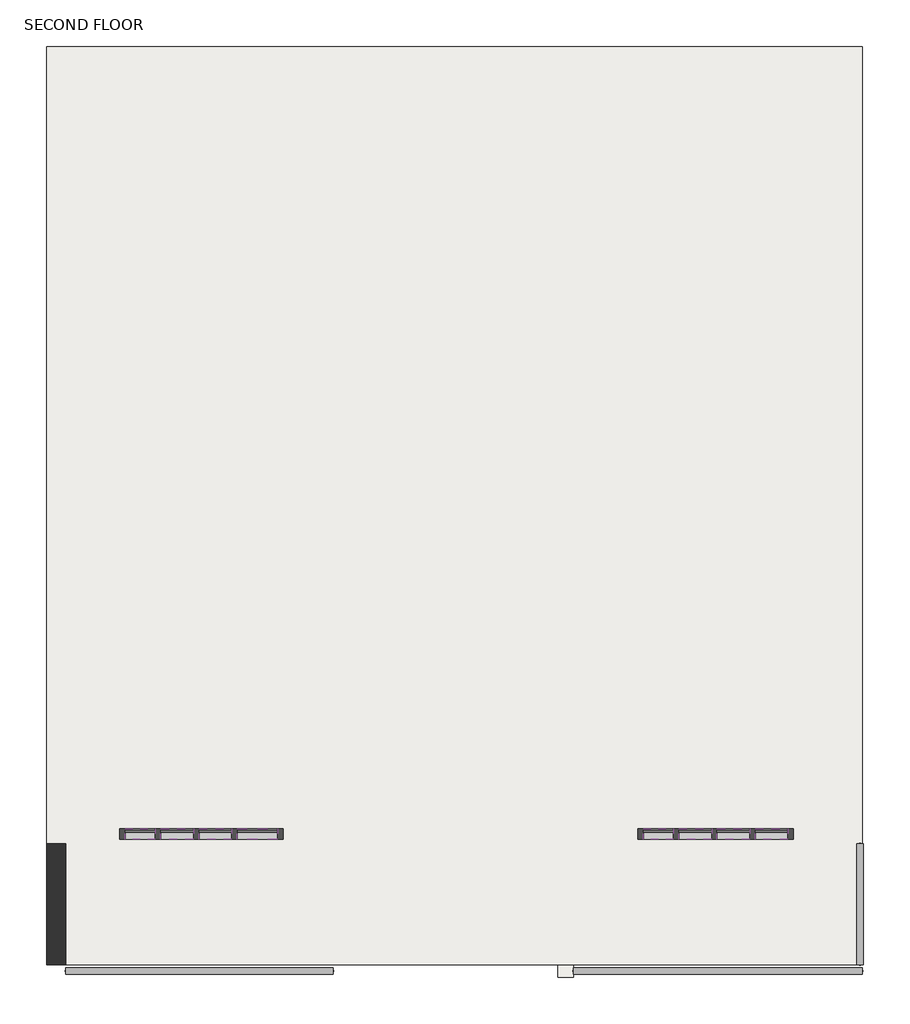
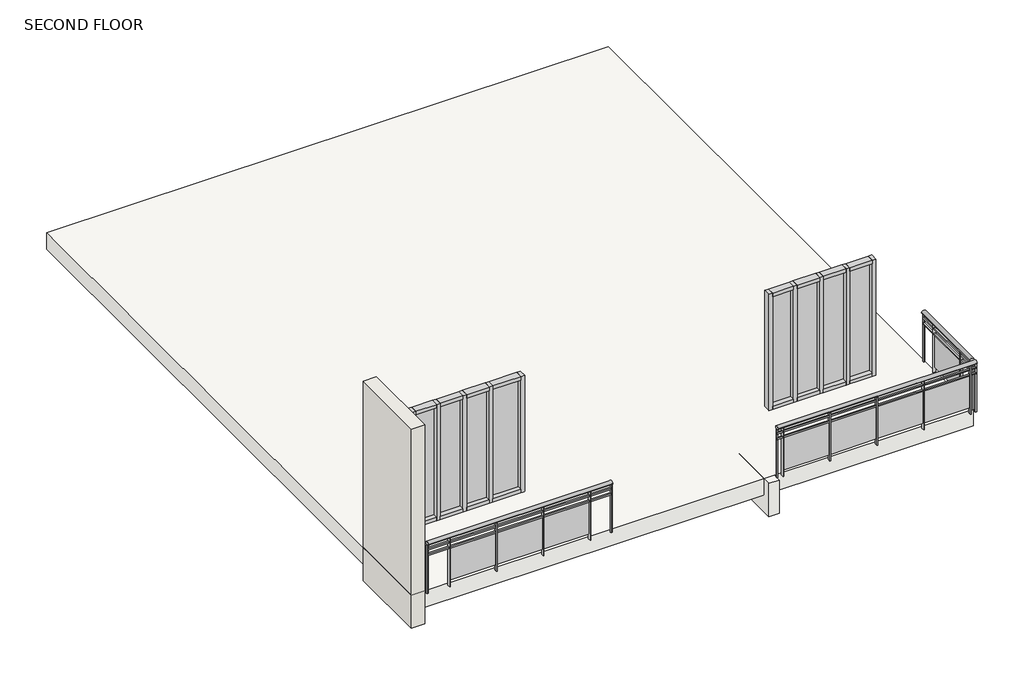
# One storey: 26 members, 8 plates, 3 railings, 2 slabs, 1 wall.
"""IFC4 building model written with IfcOpenShell, lengths in millimetres."""

from ifc_helpers import new_model, si_unit, point, frame, origin, place, context, project, spatial, polyline, ellipse_curve, trimmed, outline, extrude, transform, mapped, element, save
from ifc_brep_helpers import plane_surface, extruded_surface, advanced_brep
from components import member_3374d9b6, member_7cbddb58, member_843225dc, member_7096a90e, member_499db0bc, member_75a0f14a, system_panel_glazed_935821d8, system_panel_glazed_f3f5655f, system_panel_glazed_1490133a, system_panel_glazed_451412b5, floors_3_floors_3_f25fb9f3

model = new_model("IFC4")

# Units and contexts
model_context = context("Model", 3, world=origin())
ifc_project = project(units=[si_unit("LENGTHUNIT", "METRE", prefix="MILLI")], contexts=[model_context])

# Site, building, storey
site = spatial("IfcSite", under=ifc_project)
building = spatial("IfcBuilding", under=site)
storey = spatial("IfcBuildingStorey", under=building, Name="SECOND FLOOR", Elevation=6096.0)

# Members
placement = place(None, origin())
member_shape = member_3374d9b6(model_context)
element("IfcMember", 1, ObjectType="Rectangular Mullion : 2.5\" x 5\" rectangular", at=placement, inside=storey, context=model_context, shape_type="MappedRepresentation", body=[
    mapped(member_shape, transform((-3493.058803, -508.3464931, 6096.0), x_axis=(1.0, 0.0, 0.0), y_axis=(0.0, -1.0, 0.0), z_axis=(0.0, 0.0, -1.0))),
])
element("IfcMember", 2, ObjectType="Rectangular Mullion : 2.5\" x 5\" rectangular", at=placement, inside=storey, context=model_context, shape_type="MappedRepresentation", body=[
    mapped(member_shape, transform((2606.0769214, -508.3464931, 6096.0), x_axis=(1.0, 0.0, 0.0), y_axis=(0.0, -1.0, 0.0), z_axis=(0.0, 0.0, -1.0))),
])
element("IfcMember", 3, ObjectType="Rectangular Mullion : 2.5\" x 5\" rectangular", at=placement, inside=storey, context=model_context, shape_type="MappedRepresentation", body=[
    mapped(member_shape, transform((-5445.7230786, -508.3464931, 8229.6), x_axis=(-1.0, 0.0, 0.0), y_axis=(0.0, -1.0, 0.0), z_axis=(0.0, 0.0, 1.0))),
])
element("IfcMember", 4, ObjectType="Rectangular Mullion : 2.5\" x 5\" rectangular", at=placement, inside=storey, context=model_context, shape_type="MappedRepresentation", body=[
    mapped(member_shape, transform((748.741197, -508.3464931, 8229.6), x_axis=(-1.0, 0.0, 0.0), y_axis=(0.0, -1.0, 0.0), z_axis=(0.0, 0.0, 1.0))),
])
member_2_shape = member_7cbddb58(model_context)
element("IfcMember", 5, ObjectType="Rectangular Mullion : 2.5\" x 5\" rectangular", at=placement, inside=storey, context=model_context, shape_type="MappedRepresentation", body=[
    mapped(member_2_shape, transform((-4988.5230786, -508.3464931, 6096.0), x_axis=(1.0, 0.0, 0.0), y_axis=(0.0, -1.0, 0.0), z_axis=(0.0, 0.0, -1.0))),
])
element("IfcMember", 6, ObjectType="Rectangular Mullion : 2.5\" x 5\" rectangular", at=placement, inside=storey, context=model_context, shape_type="MappedRepresentation", body=[
    mapped(member_2_shape, transform((-4531.3230786, -508.3464931, 6096.0), x_axis=(1.0, 0.0, 0.0), y_axis=(0.0, -1.0, 0.0), z_axis=(0.0, 0.0, -1.0))),
])
element("IfcMember", 7, ObjectType="Rectangular Mullion : 2.5\" x 5\" rectangular", at=placement, inside=storey, context=model_context, shape_type="MappedRepresentation", body=[
    mapped(member_2_shape, transform((-4074.1230786, -508.3464931, 6096.0), x_axis=(1.0, 0.0, 0.0), y_axis=(0.0, -1.0, 0.0), z_axis=(0.0, 0.0, -1.0))),
])
element("IfcMember", 8, ObjectType="Rectangular Mullion : 2.5\" x 5\" rectangular", at=placement, inside=storey, context=model_context, shape_type="MappedRepresentation", body=[
    mapped(member_2_shape, transform((1205.941197, -508.3464931, 6096.0), x_axis=(1.0, 0.0, 0.0), y_axis=(0.0, -1.0, 0.0), z_axis=(0.0, 0.0, -1.0))),
])
element("IfcMember", 9, ObjectType="Rectangular Mullion : 2.5\" x 5\" rectangular", at=placement, inside=storey, context=model_context, shape_type="MappedRepresentation", body=[
    mapped(member_2_shape, transform((1663.141197, -508.3464931, 6096.0), x_axis=(1.0, 0.0, 0.0), y_axis=(0.0, -1.0, 0.0), z_axis=(0.0, 0.0, -1.0))),
])
element("IfcMember", 10, ObjectType="Rectangular Mullion : 2.5\" x 5\" rectangular", at=placement, inside=storey, context=model_context, shape_type="MappedRepresentation", body=[
    mapped(member_2_shape, transform((2120.341197, -508.3464931, 6096.0), x_axis=(1.0, 0.0, 0.0), y_axis=(0.0, -1.0, 0.0), z_axis=(0.0, 0.0, -1.0))),
])
member_3_shape = member_843225dc(model_context)
element("IfcMember", 11, ObjectType="Rectangular Mullion : 2.5\" x 5\" rectangular", at=placement, inside=storey, context=model_context, shape_type="MappedRepresentation", body=[
    mapped(member_3_shape, transform((-5382.2230786, -508.3464931, 6096.0), x_axis=(0.0, 0.0, -1.0), y_axis=(0.0, -1.0, 0.0), z_axis=(-1.0, 0.0, 0.0))),
])
element("IfcMember", 12, ObjectType="Rectangular Mullion : 2.5\" x 5\" rectangular", at=placement, inside=storey, context=model_context, shape_type="MappedRepresentation", body=[
    mapped(member_3_shape, transform((812.241197, -508.3464931, 6096.0), x_axis=(0.0, 0.0, -1.0), y_axis=(0.0, -1.0, 0.0), z_axis=(-1.0, 0.0, 0.0))),
])
element("IfcMember", 13, ObjectType="Rectangular Mullion : 2.5\" x 5\" rectangular", at=placement, inside=storey, context=model_context, shape_type="MappedRepresentation", body=[
    mapped(member_3_shape, transform((-5020.2730786, -508.3464931, 8229.6), x_axis=(0.0, 0.0, 1.0), y_axis=(0.0, -1.0, 0.0), z_axis=(1.0, 0.0, 0.0))),
])
element("IfcMember", 14, ObjectType="Rectangular Mullion : 2.5\" x 5\" rectangular", at=placement, inside=storey, context=model_context, shape_type="MappedRepresentation", body=[
    mapped(member_3_shape, transform((1174.191197, -508.3464931, 8229.6), x_axis=(0.0, 0.0, 1.0), y_axis=(0.0, -1.0, 0.0), z_axis=(1.0, 0.0, 0.0))),
])
member_4_shape = member_7096a90e(model_context)
element("IfcMember", 15, ObjectType="Rectangular Mullion : 2.5\" x 5\" rectangular", at=placement, inside=storey, context=model_context, shape_type="MappedRepresentation", body=[
    mapped(member_4_shape, transform((-4956.7730786, -508.3464931, 6096.0), x_axis=(0.0, 0.0, -1.0), y_axis=(0.0, -1.0, 0.0), z_axis=(-1.0, 0.0, 0.0))),
])
element("IfcMember", 16, ObjectType="Rectangular Mullion : 2.5\" x 5\" rectangular", at=placement, inside=storey, context=model_context, shape_type="MappedRepresentation", body=[
    mapped(member_4_shape, transform((-4499.5730786, -508.3464931, 6096.0), x_axis=(0.0, 0.0, -1.0), y_axis=(0.0, -1.0, 0.0), z_axis=(-1.0, 0.0, 0.0))),
])
element("IfcMember", 17, ObjectType="Rectangular Mullion : 2.5\" x 5\" rectangular", at=placement, inside=storey, context=model_context, shape_type="MappedRepresentation", body=[
    mapped(member_4_shape, transform((1237.691197, -508.3464931, 6096.0), x_axis=(0.0, 0.0, -1.0), y_axis=(0.0, -1.0, 0.0), z_axis=(-1.0, 0.0, 0.0))),
])
element("IfcMember", 18, ObjectType="Rectangular Mullion : 2.5\" x 5\" rectangular", at=placement, inside=storey, context=model_context, shape_type="MappedRepresentation", body=[
    mapped(member_4_shape, transform((1694.891197, -508.3464931, 6096.0), x_axis=(0.0, 0.0, -1.0), y_axis=(0.0, -1.0, 0.0), z_axis=(-1.0, 0.0, 0.0))),
])
element("IfcMember", 19, ObjectType="Rectangular Mullion : 2.5\" x 5\" rectangular", at=placement, inside=storey, context=model_context, shape_type="MappedRepresentation", body=[
    mapped(member_4_shape, transform((-4563.0730786, -508.3464931, 8229.6), x_axis=(0.0, 0.0, 1.0), y_axis=(0.0, -1.0, 0.0), z_axis=(1.0, 0.0, 0.0))),
])
element("IfcMember", 20, ObjectType="Rectangular Mullion : 2.5\" x 5\" rectangular", at=placement, inside=storey, context=model_context, shape_type="MappedRepresentation", body=[
    mapped(member_4_shape, transform((-4105.8730786, -508.3464931, 8229.6), x_axis=(0.0, 0.0, 1.0), y_axis=(0.0, -1.0, 0.0), z_axis=(1.0, 0.0, 0.0))),
])
element("IfcMember", 21, ObjectType="Rectangular Mullion : 2.5\" x 5\" rectangular", at=placement, inside=storey, context=model_context, shape_type="MappedRepresentation", body=[
    mapped(member_4_shape, transform((1631.391197, -508.3464931, 8229.6), x_axis=(0.0, 0.0, 1.0), y_axis=(0.0, -1.0, 0.0), z_axis=(1.0, 0.0, 0.0))),
])
element("IfcMember", 22, ObjectType="Rectangular Mullion : 2.5\" x 5\" rectangular", at=placement, inside=storey, context=model_context, shape_type="MappedRepresentation", body=[
    mapped(member_4_shape, transform((2088.591197, -508.3464931, 8229.6), x_axis=(0.0, 0.0, 1.0), y_axis=(0.0, -1.0, 0.0), z_axis=(1.0, 0.0, 0.0))),
])
member_5_shape = member_499db0bc(model_context)
element("IfcMember", 23, ObjectType="Rectangular Mullion : 2.5\" x 5\" rectangular", at=placement, inside=storey, context=model_context, shape_type="MappedRepresentation", body=[
    mapped(member_5_shape, transform((-3556.558803, -508.3464931, 8229.6), x_axis=(0.0, 0.0, 1.0), y_axis=(0.0, -1.0, 0.0), z_axis=(1.0, 0.0, 0.0))),
])
element("IfcMember", 24, ObjectType="Rectangular Mullion : 2.5\" x 5\" rectangular", at=placement, inside=storey, context=model_context, shape_type="MappedRepresentation", body=[
    mapped(member_5_shape, transform((-4042.3730786, -508.3464931, 6096.0), x_axis=(0.0, 0.0, -1.0), y_axis=(0.0, -1.0, 0.0), z_axis=(-1.0, 0.0, 0.0))),
])
member_6_shape = member_75a0f14a(model_context)
element("IfcMember", 25, ObjectType="Rectangular Mullion : 2.5\" x 5\" rectangular", at=placement, inside=storey, context=model_context, shape_type="MappedRepresentation", body=[
    mapped(member_6_shape, transform((2542.5769214, -508.3464931, 8229.6), x_axis=(0.0, 0.0, 1.0), y_axis=(0.0, -1.0, 0.0), z_axis=(1.0, 0.0, 0.0))),
])
element("IfcMember", 26, ObjectType="Rectangular Mullion : 2.5\" x 5\" rectangular", at=placement, inside=storey, context=model_context, shape_type="MappedRepresentation", body=[
    mapped(member_6_shape, transform((2152.091197, -508.3464931, 6096.0), x_axis=(0.0, 0.0, -1.0), y_axis=(0.0, -1.0, 0.0), z_axis=(-1.0, 0.0, 0.0))),
])

# Plates
system_panel_glazed_shape = system_panel_glazed_935821d8(model_context)
element("IfcPlate", 27, ObjectType="System Panel : Glazed", at=placement, inside=storey, context=model_context, shape_type="MappedRepresentation", body=[
    mapped(system_panel_glazed_shape, transform((-5201.2480786, -508.3464931, 6159.5), x_axis=(1.0, 0.0, 0.0), y_axis=(0.0, 1.0, 0.0), z_axis=(0.0, 0.0, 1.0))),
])
element("IfcPlate", 28, ObjectType="System Panel : Glazed", at=placement, inside=storey, context=model_context, shape_type="MappedRepresentation", body=[
    mapped(system_panel_glazed_shape, transform((993.216197, -508.3464931, 6159.5), x_axis=(1.0, 0.0, 0.0), y_axis=(0.0, 1.0, 0.0), z_axis=(0.0, 0.0, 1.0))),
])
system_panel_glazed_2_shape = system_panel_glazed_f3f5655f(model_context)
element("IfcPlate", 29, ObjectType="System Panel : Glazed", at=placement, inside=storey, context=model_context, shape_type="MappedRepresentation", body=[
    mapped(system_panel_glazed_2_shape, transform((-4759.9230786, -508.3464931, 6159.5), x_axis=(1.0, 0.0, 0.0), y_axis=(0.0, 1.0, 0.0), z_axis=(0.0, 0.0, 1.0))),
])
element("IfcPlate", 30, ObjectType="System Panel : Glazed", at=placement, inside=storey, context=model_context, shape_type="MappedRepresentation", body=[
    mapped(system_panel_glazed_2_shape, transform((-4302.7230786, -508.3464931, 6159.5), x_axis=(1.0, 0.0, 0.0), y_axis=(0.0, 1.0, 0.0), z_axis=(0.0, 0.0, 1.0))),
])
element("IfcPlate", 31, ObjectType="System Panel : Glazed", at=placement, inside=storey, context=model_context, shape_type="MappedRepresentation", body=[
    mapped(system_panel_glazed_2_shape, transform((1434.541197, -508.3464931, 6159.5), x_axis=(1.0, 0.0, 0.0), y_axis=(0.0, 1.0, 0.0), z_axis=(0.0, 0.0, 1.0))),
])
element("IfcPlate", 32, ObjectType="System Panel : Glazed", at=placement, inside=storey, context=model_context, shape_type="MappedRepresentation", body=[
    mapped(system_panel_glazed_2_shape, transform((1891.741197, -508.3464931, 6159.5), x_axis=(1.0, 0.0, 0.0), y_axis=(0.0, 1.0, 0.0), z_axis=(0.0, 0.0, 1.0))),
])
system_panel_glazed_3_shape = system_panel_glazed_1490133a(model_context)
element("IfcPlate", 33, ObjectType="System Panel : Glazed", at=placement, inside=storey, context=model_context, shape_type="MappedRepresentation", body=[
    mapped(system_panel_glazed_3_shape, transform((-3799.4659408, -508.3464931, 6159.5), x_axis=(1.0, 0.0, 0.0), y_axis=(0.0, 1.0, 0.0), z_axis=(0.0, 0.0, 1.0))),
])
system_panel_glazed_4_shape = system_panel_glazed_451412b5(model_context)
element("IfcPlate", 34, ObjectType="System Panel : Glazed", at=placement, inside=storey, context=model_context, shape_type="MappedRepresentation", body=[
    mapped(system_panel_glazed_4_shape, transform((2347.3340592, -508.3464931, 6159.5), x_axis=(1.0, 0.0, 0.0), y_axis=(0.0, 1.0, 0.0), z_axis=(0.0, 0.0, 1.0))),
])

# Railings
element("IfcRailing", 35, ObjectType="Glass Panel - Bottom Fill", at=placement, inside=storey, context=model_context, shape_type="SolidModel", body=[
    advanced_brep(
    [(-6093.4230786, -2108.5464178, 7010.4), (-6093.4230786, -2184.7464178, 7010.4), (-2893.0230786, -2108.5464178, 7010.4), (-2893.0230786, -2184.7464178, 7010.4)],
    [
        (0, 1, ellipse_curve(frame((-6093.4230786, -2146.6464178, 7010.4), z_axis=(-1.0, 0.0, 0.0), x_axis=(0.0, -1.0, 0.0)), 38.1, 28.575)),
        (1, 0, ellipse_curve(frame((-6093.4230786, -2146.6464178, 7010.4), z_axis=(-1.0, 0.0, 0.0), x_axis=(0.0, -1.0, 0.0)), 38.1, 28.575)),
        (2, 3, ellipse_curve(frame((-2893.0230786, -2146.6464178, 7010.4), z_axis=(1.0, 0.0, 0.0), x_axis=(0.0, -1.0, 0.0)), 38.1, 28.575)),
        (3, 2, ellipse_curve(frame((-2893.0230786, -2146.6464178, 7010.4), z_axis=(1.0, 0.0, 0.0), x_axis=(0.0, -1.0, 0.0)), 38.1, 28.575)),
        (0, 2),
        (3, 1),
    ],
    [
        plane_surface(frame((-6093.4230786, -2146.6464178, 7010.4), z_axis=(-1.0, 0.0, 0.0), x_axis=(0.0, 1.0, 0.0))),
        plane_surface(frame((-2893.0230786, -2146.6464178, 7010.4), z_axis=(1.0, 0.0, 0.0), x_axis=(0.0, 1.0, 0.0))),
        extruded_surface(trimmed(ellipse_curve(frame((-2893.0230786, -2146.6464178, 7010.4), z_axis=(-1.0, 0.0, 0.0), x_axis=(0.0, -1.0, 0.0)), 38.1, 28.575), [point((-2893.0230786, -2108.5464178, 7010.4))], [point((-2893.0230786, -2184.7464178, 7010.4))], True, "CARTESIAN"), (-3200.3999999999996, 0.0, 0.0), 3200.3999999999996),
        extruded_surface(trimmed(ellipse_curve(frame((-2893.0230786, -2146.6464178, 7010.4), z_axis=(-1.0, 0.0, 0.0), x_axis=(0.0, -1.0, 0.0)), 38.1, 28.575), [point((-2893.0230786, -2184.7464178, 7010.4))], [point((-2893.0230786, -2108.5464178, 7010.4))], True, "CARTESIAN"), (-3200.3999999999996, 0.0, 0.0), 3200.3999999999996),
    ],
    [
        (0, [[1, 2]]),
        (1, [[3, 4]]),
        (2, [[-1, 5, -4, 6]]),
        (3, [[-2, -6, -3, -5]]),
    ],
),
    extrude(outline(polyline([(-6093.4230786, -2159.3464178), (-6093.4230786, -2133.9464178), (-2893.0230786, -2133.9464178), (-2893.0230786, -2159.3464178), (-6093.4230786, -2159.3464178)])), frame((0.0, 0.0, 6896.1), z_axis=(0.0, 0.0, 1.0), x_axis=(1.0, 0.0, 0.0)), (0.0, 0.0, 1.0), 25.4),
    extrude(outline(polyline([(-6093.4230786, -2159.3464178), (-6093.4230786, -2133.9464178), (-2893.0230786, -2133.9464178), (-2893.0230786, -2159.3464178), (-6093.4230786, -2159.3464178)])), frame((0.0, 0.0, 6794.5), z_axis=(0.0, 0.0, 1.0), x_axis=(1.0, 0.0, 0.0)), (0.0, 0.0, 1.0), 25.4),
    extrude(outline(polyline([(-3280.3730786, -2172.0464178), (-3280.3730786, -2121.2464178), (-3267.6730786, -2121.2464178), (-3267.6730786, -2172.0464178), (-3280.3730786, -2172.0464178)])), frame((0.0, 0.0, 6096.0), z_axis=(0.0, 0.0, 1.0), x_axis=(1.0, 0.0, 0.0)), (0.0, 0.0, 1.0), 885.6788223),
    extrude(outline(polyline([(-4086.8230786, -2140.1112608), (-3274.0230786, -2140.1112608), (-3274.0230786, -2146.4612608), (-4086.8230786, -2146.4612608), (-4086.8230786, -2140.1112608)])), frame((0.0, 0.0, 6197.6), z_axis=(0.0, 0.0, 1.0), x_axis=(1.0, 0.0, 0.0)), (0.0, 0.0, 1.0), 596.9),
    extrude(outline(polyline([(-4093.1730786, -2172.0464178), (-4093.1730786, -2121.2464178), (-4080.4730786, -2121.2464178), (-4080.4730786, -2172.0464178), (-4093.1730786, -2172.0464178)])), frame((0.0, 0.0, 6096.0), z_axis=(0.0, 0.0, 1.0), x_axis=(1.0, 0.0, 0.0)), (0.0, 0.0, 1.0), 885.6788223),
    extrude(outline(polyline([(-4899.6230786, -2140.1112608), (-4086.8230786, -2140.1112608), (-4086.8230786, -2146.4612608), (-4899.6230786, -2146.4612608), (-4899.6230786, -2140.1112608)])), frame((0.0, 0.0, 6197.6), z_axis=(0.0, 0.0, 1.0), x_axis=(1.0, 0.0, 0.0)), (0.0, 0.0, 1.0), 596.9),
    extrude(outline(polyline([(-4905.9730786, -2172.0464178), (-4905.9730786, -2121.2464178), (-4893.2730786, -2121.2464178), (-4893.2730786, -2172.0464178), (-4905.9730786, -2172.0464178)])), frame((0.0, 0.0, 6096.0), z_axis=(0.0, 0.0, 1.0), x_axis=(1.0, 0.0, 0.0)), (0.0, 0.0, 1.0), 885.6788223),
    extrude(outline(polyline([(-5712.4230786, -2140.1112608), (-4899.6230786, -2140.1112608), (-4899.6230786, -2146.4612608), (-5712.4230786, -2146.4612608), (-5712.4230786, -2140.1112608)])), frame((0.0, 0.0, 6197.6), z_axis=(0.0, 0.0, 1.0), x_axis=(1.0, 0.0, 0.0)), (0.0, 0.0, 1.0), 596.9),
    extrude(outline(polyline([(-5718.7730786, -2172.0464178), (-5718.7730786, -2121.2464178), (-5706.0730786, -2121.2464178), (-5706.0730786, -2172.0464178), (-5718.7730786, -2172.0464178)])), frame((0.0, 0.0, 6096.0), z_axis=(0.0, 0.0, 1.0), x_axis=(1.0, 0.0, 0.0)), (0.0, 0.0, 1.0), 885.6788223),
    extrude(outline(polyline([(-2905.7230786, -2156.1714178), (-2905.7230786, -2137.1214178), (-2886.6730786, -2137.1214178), (-2886.6730786, -2156.1714178), (-2905.7230786, -2156.1714178)])), frame((0.0, 0.0, 6096.0), z_axis=(0.0, 0.0, 1.0), x_axis=(1.0, 0.0, 0.0)), (0.0, 0.0, 1.0), 885.6788223),
    extrude(outline(polyline([(-6099.7730786, -2156.1714178), (-6099.7730786, -2137.1214178), (-6080.7230786, -2137.1214178), (-6080.7230786, -2156.1714178), (-6099.7730786, -2156.1714178)])), frame((0.0, 0.0, 6096.0), z_axis=(0.0, 0.0, 1.0), x_axis=(1.0, 0.0, 0.0)), (0.0, 0.0, 1.0), 885.6788223),
])
element("IfcRailing", 36, ObjectType="Glass Panel - Bottom Fill", at=placement, inside=storey, context=model_context, shape_type="SolidModel", body=[
    advanced_brep(
    [(-22.6504261, -2108.5464178, 7010.4), (-22.6504261, -2184.7464178, 7010.4), (3431.5769214, -2108.5464178, 7010.4), (3431.5769214, -2184.7464178, 7010.4)],
    [
        (0, 1, ellipse_curve(frame((-22.6504261, -2146.6464178, 7010.4), z_axis=(-1.0, 0.0, 0.0), x_axis=(0.0, -1.0, 0.0)), 38.1, 28.575)),
        (1, 0, ellipse_curve(frame((-22.6504261, -2146.6464178, 7010.4), z_axis=(-1.0, 0.0, 0.0), x_axis=(0.0, -1.0, 0.0)), 38.1, 28.575)),
        (2, 3, ellipse_curve(frame((3431.5769214, -2146.6464178, 7010.4), z_axis=(1.0, 0.0, 0.0), x_axis=(0.0, -1.0, 0.0)), 38.1, 28.575)),
        (3, 2, ellipse_curve(frame((3431.5769214, -2146.6464178, 7010.4), z_axis=(1.0, 0.0, 0.0), x_axis=(0.0, -1.0, 0.0)), 38.1, 28.575)),
        (0, 2),
        (3, 1),
    ],
    [
        plane_surface(frame((-22.6504261, -2146.6464178, 7010.4), z_axis=(-1.0, 0.0, 0.0), x_axis=(0.0, 1.0, 0.0))),
        plane_surface(frame((3431.5769214, -2146.6464178, 7010.4), z_axis=(1.0, 0.0, 0.0), x_axis=(0.0, 1.0, 0.0))),
        extruded_surface(trimmed(ellipse_curve(frame((3431.5769214, -2146.6464178, 7010.4), z_axis=(-1.0, 0.0, 0.0), x_axis=(0.0, -1.0, 0.0)), 38.1, 28.575), [point((3431.5769214, -2108.5464178, 7010.4))], [point((3431.5769214, -2184.7464178, 7010.4))], True, "CARTESIAN"), (-3454.2273475, 0.0, 0.0), 3454.2273475),
        extruded_surface(trimmed(ellipse_curve(frame((3431.5769214, -2146.6464178, 7010.4), z_axis=(-1.0, 0.0, 0.0), x_axis=(0.0, -1.0, 0.0)), 38.1, 28.575), [point((3431.5769214, -2184.7464178, 7010.4))], [point((3431.5769214, -2108.5464178, 7010.4))], True, "CARTESIAN"), (-3454.2273475, 0.0, 0.0), 3454.2273475),
    ],
    [
        (0, [[1, 2]]),
        (1, [[3, 4]]),
        (2, [[-1, 5, -4, 6]]),
        (3, [[-2, -6, -3, -5]]),
    ],
),
    extrude(outline(polyline([(-22.6504261, -2159.3464178), (-22.6504261, -2133.9464178), (3431.5769214, -2133.9464178), (3431.5769214, -2159.3464178), (-22.6504261, -2159.3464178)])), frame((0.0, 0.0, 6896.1), z_axis=(0.0, 0.0, 1.0), x_axis=(1.0, 0.0, 0.0)), (0.0, 0.0, 1.0), 25.4),
    extrude(outline(polyline([(-22.6504261, -2159.3464178), (-22.6504261, -2133.9464178), (3431.5769214, -2133.9464178), (3431.5769214, -2159.3464178), (-22.6504261, -2159.3464178)])), frame((0.0, 0.0, 6794.5), z_axis=(0.0, 0.0, 1.0), x_axis=(1.0, 0.0, 0.0)), (0.0, 0.0, 1.0), 25.4),
    extrude(outline(polyline([(3323.7132477, -2172.0464178), (3323.7132477, -2121.2464178), (3336.4132477, -2121.2464178), (3336.4132477, -2172.0464178), (3323.7132477, -2172.0464178)])), frame((0.0, 0.0, 6096.0), z_axis=(0.0, 0.0, 1.0), x_axis=(1.0, 0.0, 0.0)), (0.0, 0.0, 1.0), 885.6788223),
    extrude(outline(polyline([(2517.2632477, -2140.1112608), (3330.0632477, -2140.1112608), (3330.0632477, -2146.4612608), (2517.2632477, -2146.4612608), (2517.2632477, -2140.1112608)])), frame((0.0, 0.0, 6197.6), z_axis=(0.0, 0.0, 1.0), x_axis=(1.0, 0.0, 0.0)), (0.0, 0.0, 1.0), 596.9),
    extrude(outline(polyline([(2510.9132477, -2172.0464178), (2510.9132477, -2121.2464178), (2523.6132477, -2121.2464178), (2523.6132477, -2172.0464178), (2510.9132477, -2172.0464178)])), frame((0.0, 0.0, 6096.0), z_axis=(0.0, 0.0, 1.0), x_axis=(1.0, 0.0, 0.0)), (0.0, 0.0, 1.0), 885.6788223),
    extrude(outline(polyline([(1704.4632477, -2140.1112608), (2517.2632477, -2140.1112608), (2517.2632477, -2146.4612608), (1704.4632477, -2146.4612608), (1704.4632477, -2140.1112608)])), frame((0.0, 0.0, 6197.6), z_axis=(0.0, 0.0, 1.0), x_axis=(1.0, 0.0, 0.0)), (0.0, 0.0, 1.0), 596.9),
    extrude(outline(polyline([(1698.1132477, -2172.0464178), (1698.1132477, -2121.2464178), (1710.8132477, -2121.2464178), (1710.8132477, -2172.0464178), (1698.1132477, -2172.0464178)])), frame((0.0, 0.0, 6096.0), z_axis=(0.0, 0.0, 1.0), x_axis=(1.0, 0.0, 0.0)), (0.0, 0.0, 1.0), 885.6788223),
    extrude(outline(polyline([(891.6632477, -2140.1112608), (1704.4632477, -2140.1112608), (1704.4632477, -2146.4612608), (891.6632477, -2146.4612608), (891.6632477, -2140.1112608)])), frame((0.0, 0.0, 6197.6), z_axis=(0.0, 0.0, 1.0), x_axis=(1.0, 0.0, 0.0)), (0.0, 0.0, 1.0), 596.9),
    extrude(outline(polyline([(885.3132477, -2172.0464178), (885.3132477, -2121.2464178), (898.0132477, -2121.2464178), (898.0132477, -2172.0464178), (885.3132477, -2172.0464178)])), frame((0.0, 0.0, 6096.0), z_axis=(0.0, 0.0, 1.0), x_axis=(1.0, 0.0, 0.0)), (0.0, 0.0, 1.0), 885.6788223),
    extrude(outline(polyline([(78.8632477, -2140.1112608), (891.6632477, -2140.1112608), (891.6632477, -2146.4612608), (78.8632477, -2146.4612608), (78.8632477, -2140.1112608)])), frame((0.0, 0.0, 6197.6), z_axis=(0.0, 0.0, 1.0), x_axis=(1.0, 0.0, 0.0)), (0.0, 0.0, 1.0), 596.9),
    extrude(outline(polyline([(72.5132477, -2172.0464178), (72.5132477, -2121.2464178), (85.2132477, -2121.2464178), (85.2132477, -2172.0464178), (72.5132477, -2172.0464178)])), frame((0.0, 0.0, 6096.0), z_axis=(0.0, 0.0, 1.0), x_axis=(1.0, 0.0, 0.0)), (0.0, 0.0, 1.0), 885.6788223),
    extrude(outline(polyline([(3418.8769214, -2156.1714178), (3418.8769214, -2137.1214178), (3437.9269214, -2137.1214178), (3437.9269214, -2156.1714178), (3418.8769214, -2156.1714178)])), frame((0.0, 0.0, 6096.0), z_axis=(0.0, 0.0, 1.0), x_axis=(1.0, 0.0, 0.0)), (0.0, 0.0, 1.0), 885.6788223),
    extrude(outline(polyline([(-29.0004261, -2156.1714178), (-29.0004261, -2137.1214178), (-9.9504261, -2137.1214178), (-9.9504261, -2156.1714178), (-29.0004261, -2156.1714178)])), frame((0.0, 0.0, 6096.0), z_axis=(0.0, 0.0, 1.0), x_axis=(1.0, 0.0, 0.0)), (0.0, 0.0, 1.0), 885.6788223),
])
element("IfcRailing", 37, ObjectType="Glass Panel - Bottom Fill", at=placement, inside=storey, context=model_context, shape_type="SolidModel", body=[
    advanced_brep(
    [(3444.2769214, -622.6464931, 7010.4), (3368.0769214, -622.6464931, 7010.4), (3444.2769214, -2070.4464178, 7010.4), (3368.0769214, -2070.4464178, 7010.4)],
    [
        (0, 1, ellipse_curve(frame((3406.1769214, -622.6464931, 7010.4), z_axis=(0.0, 1.0, 0.0), x_axis=(-1.0, 0.0, 0.0)), 38.1, 28.575)),
        (1, 0, ellipse_curve(frame((3406.1769214, -622.6464931, 7010.4), z_axis=(0.0, 1.0, 0.0), x_axis=(-1.0, 0.0, 0.0)), 38.1, 28.575)),
        (2, 3, ellipse_curve(frame((3406.1769214, -2070.4464178, 7010.4), z_axis=(0.0, -1.0, 0.0), x_axis=(-1.0, 0.0, 0.0)), 38.1, 28.575)),
        (3, 2, ellipse_curve(frame((3406.1769214, -2070.4464178, 7010.4), z_axis=(0.0, -1.0, 0.0), x_axis=(-1.0, 0.0, 0.0)), 38.1, 28.575)),
        (0, 2),
        (3, 1),
    ],
    [
        plane_surface(frame((3406.1769214, -622.6464931, 7010.4), z_axis=(0.0, 1.0, 0.0), x_axis=(0.0, 0.0, -1.0))),
        plane_surface(frame((3406.1769214, -2070.4464178, 7010.4), z_axis=(0.0, -1.0, 0.0), x_axis=(0.0, 0.0, -1.0))),
        extruded_surface(trimmed(ellipse_curve(frame((3406.1769214, -2070.4464178, 7010.4), z_axis=(0.0, 1.0, 0.0), x_axis=(-1.0, 0.0, 0.0)), 38.1, 28.575), [point((3444.2769214, -2070.4464178, 7010.4))], [point((3368.0769214, -2070.4464178, 7010.4))], True, "CARTESIAN"), (0.0, 1447.7999246999998, 0.0), 1447.7999246999998),
        extruded_surface(trimmed(ellipse_curve(frame((3406.1769214, -2070.4464178, 7010.4), z_axis=(0.0, 1.0, 0.0), x_axis=(-1.0, 0.0, 0.0)), 38.1, 28.575), [point((3368.0769214, -2070.4464178, 7010.4))], [point((3444.2769214, -2070.4464178, 7010.4))], True, "CARTESIAN"), (0.0, 1447.7999246999998, 0.0), 1447.7999246999998),
    ],
    [
        (0, [[1, 2]]),
        (1, [[3, 4]]),
        (2, [[-1, 5, -4, 6]]),
        (3, [[-2, -6, -3, -5]]),
    ],
),
    extrude(outline(polyline([(3393.4769214, -622.6464931), (3418.8769214, -622.6464931), (3418.8769214, -2070.4464178), (3393.4769214, -2070.4464178), (3393.4769214, -622.6464931)])), frame((0.0, 0.0, 6896.1), z_axis=(0.0, 0.0, 1.0), x_axis=(1.0, 0.0, 0.0)), (0.0, 0.0, 1.0), 25.4),
    extrude(outline(polyline([(3393.4769214, -622.6464931), (3418.8769214, -622.6464931), (3418.8769214, -2070.4464178), (3393.4769214, -2070.4464178), (3393.4769214, -622.6464931)])), frame((0.0, 0.0, 6794.5), z_axis=(0.0, 0.0, 1.0), x_axis=(1.0, 0.0, 0.0)), (0.0, 0.0, 1.0), 25.4),
    extrude(outline(polyline([(3380.7769214, -1746.5964555), (3431.5769214, -1746.5964555), (3431.5769214, -1759.2964555), (3380.7769214, -1759.2964555), (3380.7769214, -1746.5964555)])), frame((0.0, 0.0, 6096.0), z_axis=(0.0, 0.0, 1.0), x_axis=(1.0, 0.0, 0.0)), (0.0, 0.0, 1.0), 885.6788223),
    extrude(outline(polyline([(3412.7120784, -940.1464555), (3412.7120784, -1752.9464555), (3406.3620784, -1752.9464555), (3406.3620784, -940.1464555), (3412.7120784, -940.1464555)])), frame((0.0, 0.0, 6197.6), z_axis=(0.0, 0.0, 1.0), x_axis=(1.0, 0.0, 0.0)), (0.0, 0.0, 1.0), 596.9),
    extrude(outline(polyline([(3380.7769214, -933.7964555), (3431.5769214, -933.7964555), (3431.5769214, -946.4964555), (3380.7769214, -946.4964555), (3380.7769214, -933.7964555)])), frame((0.0, 0.0, 6096.0), z_axis=(0.0, 0.0, 1.0), x_axis=(1.0, 0.0, 0.0)), (0.0, 0.0, 1.0), 885.6788223),
    extrude(outline(polyline([(3396.6519214, -2057.7464178), (3415.7019214, -2057.7464178), (3415.7019214, -2076.7964178), (3396.6519214, -2076.7964178), (3396.6519214, -2057.7464178)])), frame((0.0, 0.0, 6096.0), z_axis=(0.0, 0.0, 1.0), x_axis=(1.0, 0.0, 0.0)), (0.0, 0.0, 1.0), 885.6788223),
    extrude(outline(polyline([(3396.6519214, -616.2964931), (3415.7019214, -616.2964931), (3415.7019214, -635.3464931), (3396.6519214, -635.3464931), (3396.6519214, -616.2964931)])), frame((0.0, 0.0, 6096.0), z_axis=(0.0, 0.0, 1.0), x_axis=(1.0, 0.0, 0.0)), (0.0, 0.0, 1.0), 885.6788223),
])

# Slabs
floors_3_floors_3_shape = floors_3_floors_3_f25fb9f3(model_context)
element("IfcSlab", 38, ObjectType="Floors 3 : Floors 3", at=placement, inside=storey, context=model_context, shape_type="MappedRepresentation", body=[
    mapped(floors_3_floors_3_shape, transform((0.0, 0.0, 0.0), x_axis=(1.0, 0.0, 0.0), y_axis=(0.0, 1.0, 0.0), z_axis=(0.0, 0.0, 1.0))),
])
element("IfcSlab", 39, ObjectType="Generic - 12\"", at=placement, inside=storey, context=model_context, shape_type="SweptSolid", body=[
    extrude(outline(polyline([(3431.5769214, -2070.4464178), (-6322.0230786, -2070.4464178), (-6322.0230786, 8902.3535822), (3431.5769214, 8902.3535822), (3431.5769214, -2070.4464178)])), frame((0.0, 0.0, 5791.2), z_axis=(0.0, 0.0, 1.0), x_axis=(1.0, 0.0, 0.0)), (0.0, 0.0, 1.0), 304.8),
])

# Wall
element("IfcWall", 40, ObjectType="9\"", at=placement, inside=storey, context=model_context, shape_type="SweptSolid", body=[
    extrude(outline(polyline([(-6322.0230786, -2070.4464178), (-6322.0230786, -622.6464931), (-6093.4230786, -622.6464931), (-6093.4230786, -2070.4464178), (-6322.0230786, -2070.4464178)])), frame((0.0, 0.0, 5486.4), z_axis=(0.0, 0.0, 1.0), x_axis=(1.0, 0.0, 0.0)), (0.0, 0.0, 1.0), 3657.6),
])

save(model, "model.ifc")

# Revit data of these elements
# Type "Rectangular Mullion : 2.5\" x 5\" rectangular"
#   built-in parameter 1007304 = 0.416667 (stored number, unit not read)
#   built-in parameter 1007301 = 0.104167 (stored number, unit not read)
#   built-in parameter 1007300 = 0.104167 (stored number, unit not read)
# Type "System Panel : Glazed"
#   Construction Type Id = "GSP4R"
#   Analytic Construction = "1/8 in Pilkington single glazing"
#   Visual Light Transmittance = 0.9
#   Solar Heat Gain Coefficient = 0.86
#   Heat Transfer Coefficient (U) = 1.18115 BTU/(h·ft²·°F)
#   Define Thermal Properties by = 1
# Type "Glass Panel - Bottom Fill"
#   Assembly Code = "C2010400"
#   built-in parameter 1008612 = 0.0416667 (stored number, unit not read)
#   built-in parameter 1008611 = 0.0416667 (stored number, unit not read)
#   built-in parameter 1008609 = 0.333333 (stored number, unit not read)
#   built-in parameter 1008604 = 0.166667 (stored number, unit not read)
#   built-in parameter 1008603 = 0.166667 (stored number, unit not read)
#   Railing Height = 3' - 0"
#   built-in parameter 1008630 = 2
#   built-in parameter 1008610 = 2
#   built-in parameter 1008618 = Baluster - Square : 3/4"
# Type "Generic - 12\""
#   Assembly Code = "B1010"
#   Function = 0
#   Layers, outside or top first: 1' - 0" no material (function 1)
# Type "9\""
#   Assembly Code = "B2010"
#   Layers, outside or top first: 0' - 9" no material (function 1)
# Elements 1, 2, 3, 4, 5, 6, 7, 8, 9, 10, 11, 12, 13, 14, 15, 16, 17, 18, 19, 20, 21, 22, 23, 24, 25, 26 (IfcMember, "Rectangular Mullion : 2.5\" x 5\" rectangular")
#   Phase Created = New Construction
#   Materials on its faces: "Aluminum"
# Elements 27, 28, 29, 30, 31, 32, 33, 34 (IfcPlate, "System Panel : Glazed")
#   Phase Created = New Construction
#   Materials on its faces: "Glass"
# Elements 35, 36, 37 (IfcRailing, "Glass Panel - Bottom Fill")
#   Phase Created = New Construction
#   Materials on its faces: "Glass"
# Element 38 (IfcSlab, "Floors 3 : Floors 3")
#   Phase Created = New Construction
#   Materials on its faces: "Default Floor"
# Element 39 (IfcSlab, "Generic - 12\"")
#   Height Offset From Level = 0' - 0"
#   Phase Created = New Construction
#   Materials on its faces: "Default Floor", "1 wall"
# Element 40 (IfcWall, "9\"")
#   built-in parameter 1001111 = -2' - 0"
#   Top Offset = 0' - 0"
#   Base Offset = -2' - 0"
#   Unconnected Height = 12' - 0"
#   wall height = 12' - 0"
#   Phase Created = New Construction
#   Base Constraint = SECOND FLOOR
#   Materials on its faces: "Default Wall", "1 wall"
# Materials
#   "Aluminum": class "Metal", colour RGB 247 247 247, transparency 0, Description = "Aluminum 6061", Cost = 0
#   "Glass": class "Glass", colour RGB 0 128 192, transparency 0.75, Description = "Soda Lime Glass", Cost = 0
#   "Default Floor": colour RGB 128 128 128, transparency 0, Cost = 0
#   "1 wall": class "Generic", colour RGB 244 245 241, transparency 0, Cost = 0
#   "Default Wall": colour RGB 128 128 128, transparency 0, Cost = 0
